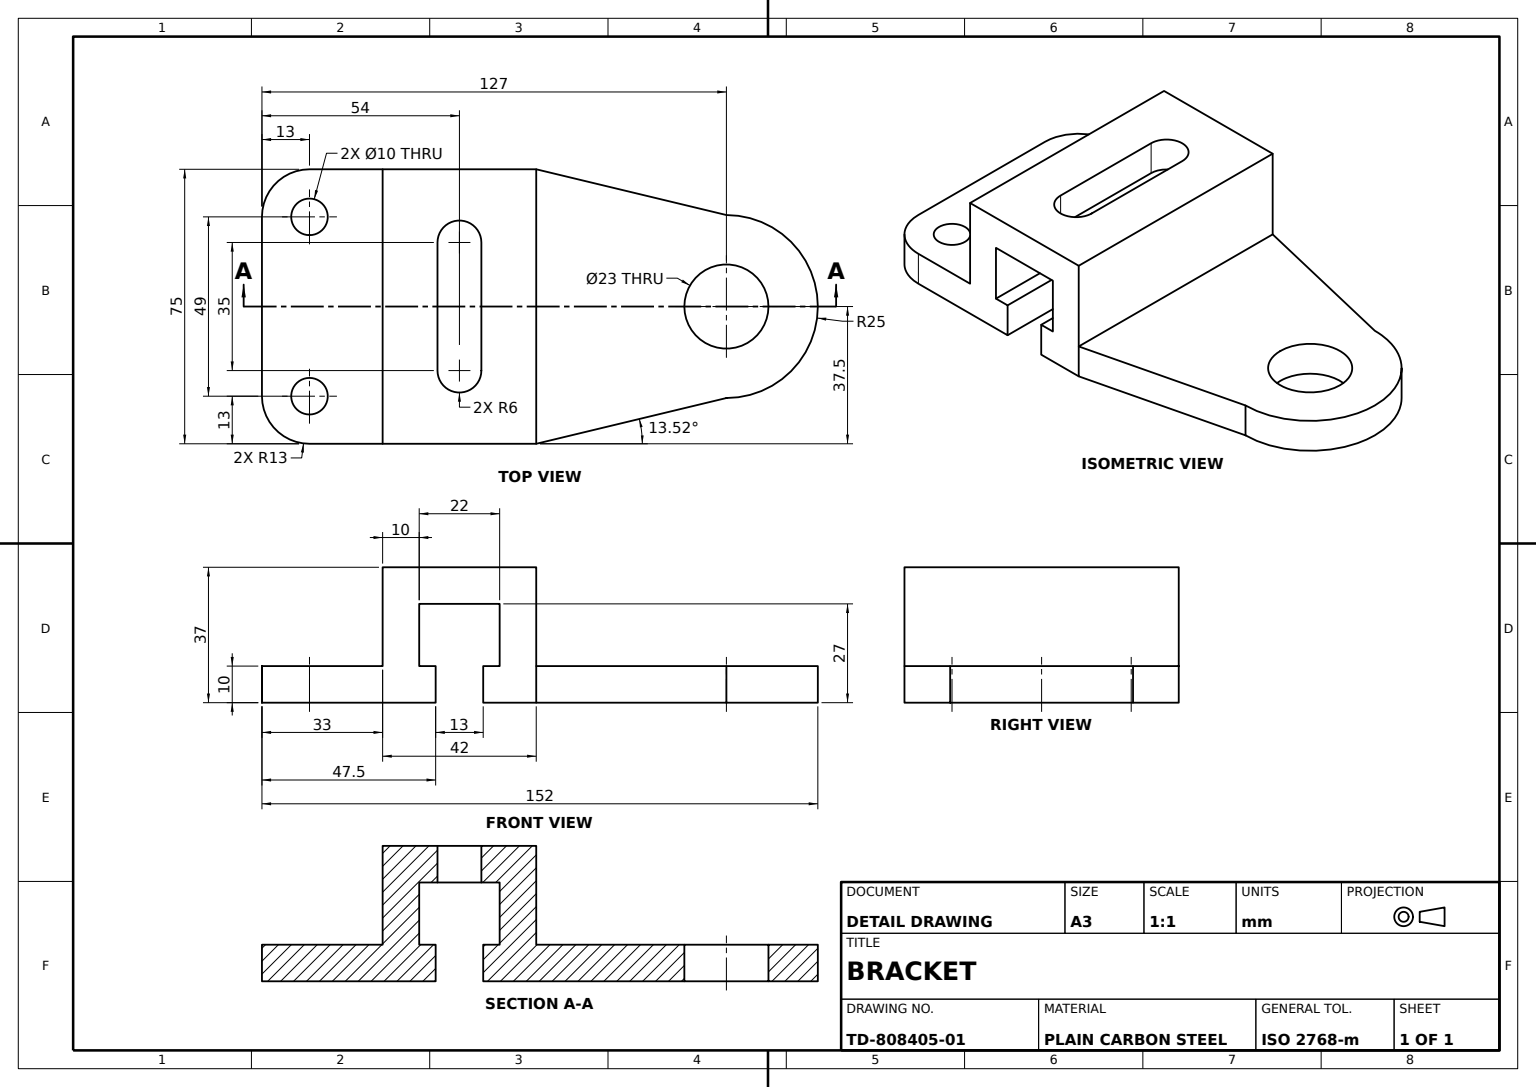
SolidWorks part; units mm, degrees
material "Plain Carbon Steel"
ref_plane "Front Plane" through (0, 0, 0) normal (0, 0, 1) x (1, 0, 0)
ref_plane "Top Plane" through (0, 0, 0) normal (0, 1, 0) x (1, 0, 0)
ref_plane "Right Plane" through (0, 0, 0) normal (1, 0, 0) x (0, 0, -1)
sketch "Base Profile Sketch" plane through (0, 0, 0) normal (0, 0, 1) x (1, 0, 0)
  line L0 (0, 11) -> (0, 21)
  line L1 (0, 21) -> (-27, 21)
  line L2 (-27, 21) -> (-27, -21)
  line L3 (-27, -21) -> (0, -21)
  line L4 (0, -21) -> (0, -11)
  line L5 (0, -11) -> (-17, -11)
  line L6 (-17, -11) -> (-17, 11)
  line L7 (-17, 11) -> (0, 11)
  dimension "D1" = 42
  dimension "D2" = 27
  dimension "D3" = 27
  dimension "D4" = 21
  dimension "D5" = 22
  dimension "D6" = 11
  dimension "D7" = 17
extrude "Base Body" add sketch "Base Profile Sketch" along normal mid plane 75
sketch "Upper Flange Sketch" plane through (0, 0, 37.5) normal (0, 0, 1) x (1, 0, 0)
  line L0 (0, 21) -> (0, 54)
  line L1 (0, 6.5) -> (10, 6.5)
  line L2 (10, 6.5) -> (10, 21)
  line L4 (0, 21) -> (0, 6.5)
  line L5 (0, 54) -> (10, 54)
  line L6 (10, 54) -> (10, 21)
  dimension "D1" = 47.5
  dimension "D2" = 33
  dimension "D3" = 10
  dimension "D4" = 54
extrude "Upper Flange" add sketch "Upper Flange Sketch" against normal blind 75
fillet "Flange Corner Fillet R13 A" radius 13 1 edges at (5, 54, 37.5)
fillet "Flange Corner Fillet R13 B" radius 13 1 edges at (5, 54, -37.5)
sketch "Mounting Holes Sketch" plane through (0, 0, 0) normal (-1, 0, 0) x (0, 0, 1)
  circle A0 centre (24.5, 41) radius 5
  circle A1 centre (-24.5, 41) radius 5
  dimension "D1" = 10
  dimension "D2" = 10
extrude "Mounting Holes 2xØ10" cut sketch "Mounting Holes Sketch" against normal blind 75
sketch "Slot Sketch" plane through (-27, 0, 0) normal (-1, 0, 0) x (0, 0, 1)
  line L0 (37.5, 21) -> (-37.5, 21) construction
  line L2 (-17.5, 6) -> (17.5, 6)
  line L3 (-17.5, -6) -> (17.5, -6)
  arc A0 (17.5, -6) -> (17.5, 6) centre (17.5, 0) ccw
  arc A1 (-17.5, 6) -> (-17.5, -6) centre (-17.5, 0) ccw
  dimension "D1" = 6
  dimension "D2" = 17.5
  dimension "D3" = 17.5
  dimension "D4" = 15
extrude "Slot 6mm" cut sketch "Slot Sketch" against normal blind 75
sketch "Hanger Plate Sketch" plane through (0, 0, 37.5) normal (0, 0, 1) x (1, 0, 0)
  line L0 (0, -6.5) -> (0, -21)
  line L1 (0, -6.5) -> (10, -6.5)
  line L3 (10, -21) -> (10, -6.5)
  line L4 (0, -21) -> (0, -73)
  line L5 (0, -73) -> (10, -73)
  line L6 (10, -73) -> (10, -21)
  dimension "D1" = 10
  dimension "D2" = 66.5
  dimension "D3" = 73
  dimension "D4" = 10
extrude "Hanger Plate" add sketch "Hanger Plate Sketch" against normal blind 75
sketch "Taper Cut Sketch" plane through (0, 0, 0) normal (-1, 0, 0) x (0, 0, 1)
  line L0 (-37.5, -73) -> (37.5, -73) construction
  line L1 (-37.5, -21) -> (-25, -73)
  line L2 (25, -73) -> (37.5, -21)
  line L3 (37.5, -21) -> (-37.5, -21)
  line L4 (-37.5, -21) -> (-37.5, -73)
  line L5 (-37.5, -73) -> (-25, -73)
  line L6 (25, -73) -> (37.5, -73)
  line L7 (37.5, -73) -> (37.5, -21)
  circle A0 centre (0, -73) radius 25
  line M2 (-37.5, -21) -> (-37.5, -73)
  line M3 (-37.5, -73) -> (37.5, -73)
  line M4 (37.5, -73) -> (37.5, -21)
  dimension "D1" = 50
extrude "Taper Cut" cut sketch "Taper Cut Sketch" against normal blind 75 contours L2 M3 M4 | L1 M2 M3
sketch "Eye Boss Sketch" plane through (0, 0, 0) normal (-1, 0, 0) x (0, 0, 1)
  line L0 (-25, -73) -> (25, -73) construction
  circle A0 centre (0, -73) radius 25
extrude "Eye Boss" add sketch "Eye Boss Sketch" against normal blind 10
sketch "Eye Hole Sketch" plane through (0, 0, 0) normal (-1, 0, 0) x (0, 0, 1)
  circle A0 centre (0, -73) radius 11.5
  dimension "D1" = 23
extrude "Eye Hole Ø23" cut sketch "Eye Hole Sketch" against normal blind 10
